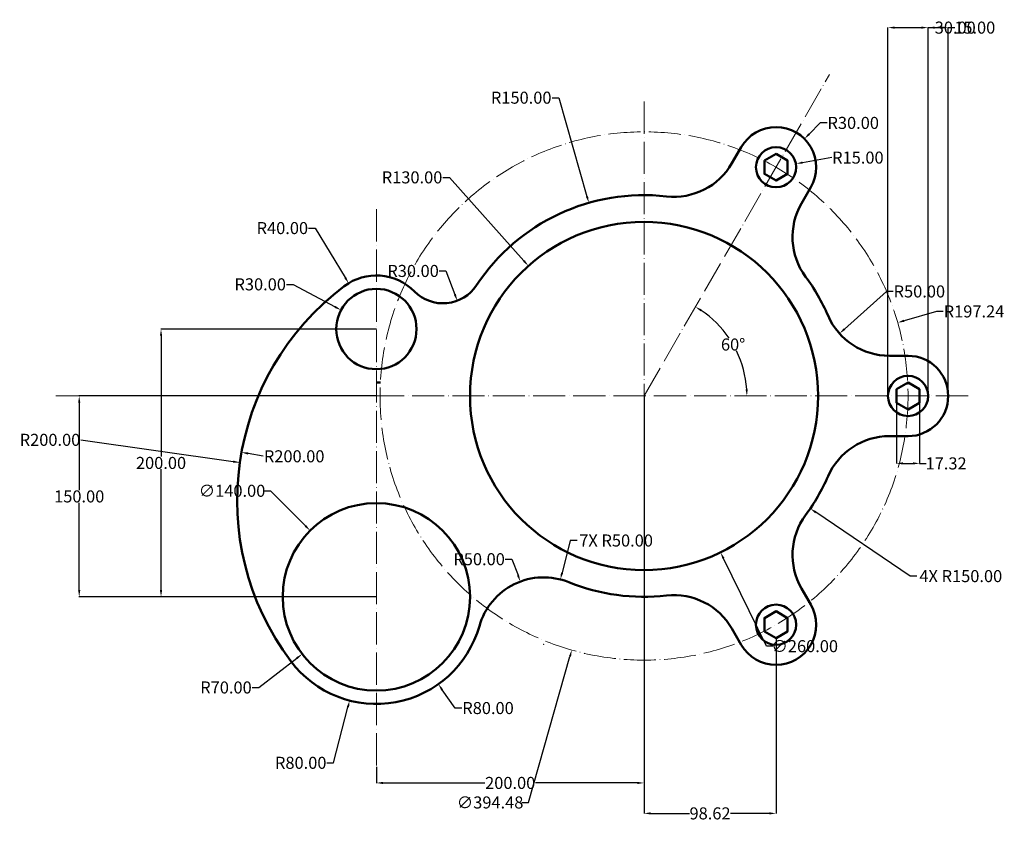
# Model space of a CAD drawing. Units: inches. Extents: x 301 to 1037, y 121 to 719.
import ezdxf

# ---------------------------------------------------------------- set-up
doc = ezdxf.new("R2010")
doc.units = ezdxf.units.IN
doc.header["$MEASUREMENT"] = 0
doc.linetypes.add('ACAD_ISO04W100', pattern=[30, 24, -3, 0, -3])
for name, color, linetype, lineweight in [('M-CNTR', 4, 'ACAD_ISO04W100', 18), ('M-DIMS', 2, 'Continuous', 25), ('M-OUTL', 7, 'Continuous', 50)]:
    doc.layers.add(name, color=color, linetype=linetype, lineweight=lineweight)
doc.styles.get("Standard").update_dxf_attribs({"font": 'arial.ttf'})
doc.dimstyles.get("Standard").update_dxf_attribs({"dimtxt": 9, "dimasz": 5, "dimexe": 0.18, "dimexo": 0.0625, "dimgap": 0.09, "dimtad": 0, "dimtih": 1, "dimtoh": 1, "dimzin": 0, "dimdsep": 46, "dimtxsty": 'Standard', "dimcen": 0.09, "dimadec": 0, "dimazin": 0, "dimtfac": 1, "dimtofl": 0, "dimtmove": 0, "dimatfit": 3, "dimfxl": 1, "dimtolj": 1, "dimtzin": 0, "dimarcsym": 0})

# ---------------------------------------------------------------- blocks, each defined once
blk = doc.blocks.new('*D1')
at = {"layer": 'Defpoints', "color": 0, "transparency": 16777216}
for p in [(567.87, 488.37), (406.98, 288.37), (567.87, 288.37)]:
    blk.add_point(p, dxfattribs=at)
at = {"layer": 'M-DIMS', "color": 0, "lineweight": -2, "transparency": 16777216}
for p, q in [((567.81, 488.37), (406.8, 488.37)), ((406.98, 483.37), (406.98, 393.06)), ((406.98, 293.37), (406.98, 383.69)), ((567.81, 288.37), (406.8, 288.37))]:
    blk.add_line(p, q, dxfattribs=at)
at = {"layer": 'M-DIMS', "color": 0, "transparency": 16777216}
for points in [[(406.15, 483.37), (407.81, 483.37), (406.98, 488.37)], [(406.15, 293.37), (407.81, 293.37), (406.98, 288.37)]]:
    blk.add_solid(points, dxfattribs=at)
at = {"layer": 'M-DIMS', "color": 0, "transparency": 16777216, "insert": (406.98, 388.37), "char_height": 9, "attachment_point": 5}
blk.add_mtext('\\A1;200.00', dxfattribs=at)
blk = doc.blocks.new('*D2')
at = {"layer": 'Defpoints', "color": 0, "transparency": 16777216}
for p in [(567.87, 438.37), (345.86, 288.37), (567.87, 288.37)]:
    blk.add_point(p, dxfattribs=at)
at = {"layer": 'M-DIMS', "color": 0, "lineweight": -2, "transparency": 16777216}
for p, q in [((567.81, 438.37), (345.68, 438.37)), ((345.86, 433.37), (345.86, 368.06)), ((345.86, 293.37), (345.86, 358.69)), ((567.81, 288.37), (345.68, 288.37))]:
    blk.add_line(p, q, dxfattribs=at)
at = {"layer": 'M-DIMS', "color": 0, "transparency": 16777216}
for points in [[(345.03, 433.37), (346.69, 433.37), (345.86, 438.37)], [(345.03, 293.37), (346.69, 293.37), (345.86, 288.37)]]:
    blk.add_solid(points, dxfattribs=at)
at = {"layer": 'M-DIMS', "color": 0, "transparency": 16777216, "insert": (345.86, 363.37), "char_height": 9, "attachment_point": 5}
blk.add_mtext('\\A1;150.00', dxfattribs=at)
blk = doc.blocks.new('*D3')
at = {"layer": 'Defpoints', "color": 0, "transparency": 16777216}
for p in [(567.87, 288.37), (512.43, 245.64)]:
    blk.add_point(p, dxfattribs=at)
at = {"layer": 'M-DIMS', "color": 0, "lineweight": -2, "transparency": 16777216}
for p, q in [((567.78, 288.37), (567.96, 288.37)), ((567.87, 288.28), (567.87, 288.46)), ((480.08, 220.7), (508.47, 242.58)), ((475.08, 220.7), (480.08, 220.7))]:
    blk.add_line(p, q, dxfattribs=at)
at = {"layer": 'M-DIMS', "color": 0, "transparency": 16777216}
blk.add_solid([(507.96, 243.24), (508.98, 241.92), (512.43, 245.64)], dxfattribs=at)
at = {"layer": 'M-DIMS', "color": 0, "transparency": 16777216, "insert": (455.51, 220.7), "char_height": 9, "attachment_point": 5}
blk.add_mtext('\\A1;R70.00', dxfattribs=at)
blk = doc.blocks.new('*D4')
at = {"layer": 'Defpoints', "color": 0, "transparency": 16777216}
for p in [(567.87, 288.37), (614.13, 223.11)]:
    blk.add_point(p, dxfattribs=at)
at = {"layer": 'M-DIMS', "color": 0, "lineweight": -2, "transparency": 16777216}
for p, q in [((567.78, 288.37), (567.96, 288.37)), ((567.87, 288.28), (567.87, 288.46)), ((626.73, 205.33), (617.02, 219.03)), ((631.73, 205.33), (626.73, 205.33))]:
    blk.add_line(p, q, dxfattribs=at)
at = {"layer": 'M-DIMS', "color": 0, "transparency": 16777216}
blk.add_solid([(617.7, 219.51), (616.34, 218.55), (614.13, 223.11)], dxfattribs=at)
at = {"layer": 'M-DIMS', "color": 0, "transparency": 16777216, "insert": (651.3, 205.33), "char_height": 9, "attachment_point": 5}
blk.add_mtext('\\A1;R80.00', dxfattribs=at)
blk = doc.blocks.new('*D5')
at = {"layer": 'Defpoints', "color": 0, "transparency": 16777216}
for p in [(767.87, 203.81), (567.87, 161.57), (767.87, 149.41)]:
    blk.add_point(p, dxfattribs=at)
at = {"layer": 'M-DIMS', "color": 0, "lineweight": -2, "transparency": 16777216}
for p, q in [((767.87, 203.75), (767.87, 149.23)), ((567.87, 161.51), (567.87, 149.23)), ((572.87, 149.41), (649.04, 149.41)), ((762.87, 149.41), (686.7, 149.41))]:
    blk.add_line(p, q, dxfattribs=at)
at = {"layer": 'M-DIMS', "color": 0, "transparency": 16777216}
for points in [[(572.87, 150.24), (572.87, 148.57), (567.87, 149.41)], [(762.87, 150.24), (762.87, 148.57), (767.87, 149.41)]]:
    blk.add_solid(points, dxfattribs=at)
at = {"layer": 'M-DIMS', "color": 0, "transparency": 16777216, "insert": (667.87, 149.41), "char_height": 9, "attachment_point": 5}
blk.add_mtext('\\A1;200.00', dxfattribs=at)
blk = doc.blocks.new('*D6')
at = {"layer": 'Defpoints', "color": 0, "transparency": 16777216}
for p in [(675.45, 299.77), (692.95, 252.94)]:
    blk.add_point(p, dxfattribs=at)
at = {"layer": 'M-DIMS', "color": 0, "lineweight": -2, "transparency": 16777216}
for p, q in [((664.2, 316.49), (669.2, 316.49)), ((669.2, 316.49), (673.7, 304.46)), ((692.86, 252.94), (693.04, 252.94)), ((692.95, 252.85), (692.95, 253.03))]:
    blk.add_line(p, q, dxfattribs=at)
at = {"layer": 'M-DIMS', "color": 0, "transparency": 16777216}
blk.add_solid([(674.48, 304.75), (672.92, 304.17), (675.45, 299.77)], dxfattribs=at)
at = {"layer": 'M-DIMS', "color": 0, "transparency": 16777216, "insert": (644.64, 316.49), "char_height": 9, "attachment_point": 5}
blk.add_mtext('\\A1;R50.00', dxfattribs=at)
blk = doc.blocks.new('*D7')
at = {"layer": 'Defpoints', "color": 0, "transparency": 16777216}
for p in [(541.43, 502.55), (567.87, 488.37)]:
    blk.add_point(p, dxfattribs=at)
at = {"layer": 'M-DIMS', "color": 0, "lineweight": -2, "transparency": 16777216}
for p, q in [((500.64, 521.73), (505.64, 521.73)), ((505.64, 521.73), (537.02, 504.91)), ((567.78, 488.37), (567.96, 488.37)), ((567.87, 488.28), (567.87, 488.46))]:
    blk.add_line(p, q, dxfattribs=at)
blk.add_arc((567.87, 488.37), 30, 151.46431, 224.53097, dxfattribs=at)
at = {"layer": 'M-DIMS', "color": 0, "transparency": 16777216}
blk.add_solid([(537.42, 505.64), (536.63, 504.17), (541.43, 502.55)], dxfattribs=at)
at = {"layer": 'M-DIMS', "color": 0, "transparency": 16777216, "insert": (481.07, 521.73), "char_height": 9, "attachment_point": 5}
blk.add_mtext('\\A1;R30.00', dxfattribs=at)
blk = doc.blocks.new('*D8')
at = {"layer": 'Defpoints', "color": 0, "transparency": 16777216}
for p in [(547.14, 522.58), (567.87, 488.37)]:
    blk.add_point(p, dxfattribs=at)
at = {"layer": 'M-DIMS', "color": 0, "lineweight": -2, "transparency": 16777216}
for p, q in [((517.2, 563.75), (522.2, 563.75)), ((522.2, 563.75), (544.55, 526.86)), ((567.78, 488.37), (567.96, 488.37)), ((567.87, 488.28), (567.87, 488.46))]:
    blk.add_line(p, q, dxfattribs=at)
at = {"layer": 'M-DIMS', "color": 0, "transparency": 16777216}
blk.add_solid([(545.26, 527.29), (543.84, 526.43), (547.14, 522.58)], dxfattribs=at)
at = {"layer": 'M-DIMS', "color": 0, "transparency": 16777216, "insert": (497.63, 563.75), "char_height": 9, "attachment_point": 5}
blk.add_mtext('\\A1;R40.00', dxfattribs=at)
blk = doc.blocks.new('*D9')
at = {"layer": 'Defpoints', "color": 0, "transparency": 16777216}
for p in [(617.67, 537.57), (628.28, 509.51)]:
    blk.add_point(p, dxfattribs=at)
at = {"layer": 'M-DIMS', "color": 0, "lineweight": -2, "transparency": 16777216}
for p, q in [((614.87, 531.74), (619.87, 531.74)), ((619.87, 531.74), (626.51, 514.18))]:
    blk.add_line(p, q, dxfattribs=at)
at = {"layer": 'M-DIMS', "color": 0, "transparency": 16777216}
blk.add_solid([(627.29, 514.48), (625.73, 513.89), (628.28, 509.51)], dxfattribs=at)
at = {"layer": 'M-DIMS', "color": 0, "transparency": 16777216, "insert": (595.3, 531.74), "char_height": 9, "attachment_point": 5}
blk.add_mtext('\\A1;R30.00', dxfattribs=at)
blk = doc.blocks.new('*D10')
at = {"layer": 'Defpoints', "color": 0, "transparency": 16777216}
for p in [(681.45, 535.49), (767.87, 438.37)]:
    blk.add_point(p, dxfattribs=at)
at = {"layer": 'M-DIMS', "color": 0, "lineweight": -2, "transparency": 16777216}
for p, q in [((617.6, 601.62), (622.6, 601.62)), ((622.6, 601.62), (678.13, 539.22)), ((767.78, 438.37), (767.96, 438.37)), ((767.87, 438.28), (767.87, 438.46))]:
    blk.add_line(p, q, dxfattribs=at)
at = {"layer": 'M-DIMS', "color": 0, "transparency": 16777216}
blk.add_solid([(678.75, 539.78), (677.5, 538.67), (681.45, 535.49)], dxfattribs=at)
at = {"layer": 'M-DIMS', "color": 0, "transparency": 16777216, "insert": (594.54, 601.62), "char_height": 9, "attachment_point": 5}
blk.add_mtext('\\A1;R130.00', dxfattribs=at)
blk = doc.blocks.new('*D11')
at = {"layer": 'Defpoints', "color": 0, "transparency": 16777216}
for p in [(467.12, 396.31), (663.87, 360.37)]:
    blk.add_point(p, dxfattribs=at)
at = {"layer": 'M-DIMS', "color": 0, "lineweight": -2, "transparency": 16777216}
blk.add_line((483.41, 393.33), (472.04, 395.41), dxfattribs=at)
at = {"layer": 'M-DIMS', "color": 0, "transparency": 16777216}
blk.add_solid([(472.19, 396.23), (471.89, 394.59), (467.12, 396.31)], dxfattribs=at)
at = {"layer": 'M-DIMS', "color": 0, "transparency": 16777216, "insert": (506.47, 393.33), "char_height": 9, "attachment_point": 5}
blk.add_mtext('\\A1;R200.00', dxfattribs=at)
blk = doc.blocks.new('*D12')
at = {"layer": 'Defpoints', "color": 0, "transparency": 16777216}
for p in [(726.62, 582.59), (767.87, 438.37)]:
    blk.add_point(p, dxfattribs=at)
at = {"layer": 'M-DIMS', "color": 0, "lineweight": -2, "transparency": 16777216}
for p, q in [((699.15, 661.13), (704.15, 661.13)), ((704.15, 661.13), (725.24, 587.4)), ((767.78, 438.37), (767.96, 438.37)), ((767.87, 438.28), (767.87, 438.46))]:
    blk.add_line(p, q, dxfattribs=at)
at = {"layer": 'M-DIMS', "color": 0, "transparency": 16777216}
blk.add_solid([(726.05, 587.63), (724.44, 587.17), (726.62, 582.59)], dxfattribs=at)
at = {"layer": 'M-DIMS', "color": 0, "transparency": 16777216, "insert": (676.09, 661.13), "char_height": 9, "attachment_point": 5}
blk.add_mtext('\\A1;R150.00', dxfattribs=at)
blk = doc.blocks.new('*U13')
for p, q in [((-0.06, 40.88), (-7.03, 28.81)), ((51.9, 10.88), (44.93, -1.19))]:
    blk.add_line(p, q)
blk.add_circle((25.92, 25.88), 15)
for centre, radius, start, end in [((25.92, 25.88), 30, 330, 150), ((-50.33, 53.81), 50, 263.57818, 330), ((88.23, -26.19), 50, 150, 216.42182)]:
    blk.add_arc(centre, radius, start, end)
blk = doc.blocks.new('*U14')
at = {"layer": 'M-OUTL', "color": 0, "linetype": 'ByBlock', "lineweight": -2, "transparency": 16777216}
blk.add_blockref('*U13', (840.57, 583.31), dxfattribs=at)
for p, rotation in [((929.74, 447.88), 300), ((857.04, 302.95), 240)]:
    blk.add_blockref('*U13', p, dxfattribs=dict(at, rotation=rotation))
blk = doc.blocks.new('*D15')
at = {"layer": 'Defpoints', "color": 0, "transparency": 16777216}
for p in [(956.45, 433.37), (973.77, 433.37), (973.77, 388.03)]:
    blk.add_point(p, dxfattribs=at)
at = {"layer": 'M-DIMS', "color": 0, "lineweight": -2, "transparency": 16777216}
for p, q in [((956.45, 433.31), (956.45, 387.85)), ((973.77, 433.31), (973.77, 387.85)), ((961.45, 388.03), (968.77, 388.03)), ((973.77, 388.03), (978.77, 388.03))]:
    blk.add_line(p, q, dxfattribs=at)
at = {"layer": 'M-DIMS', "color": 0, "transparency": 16777216}
for points in [[(961.45, 388.86), (961.45, 387.2), (956.45, 388.03)], [(968.77, 388.86), (968.77, 387.2), (973.77, 388.03)]]:
    blk.add_solid(points, dxfattribs=at)
at = {"layer": 'M-DIMS', "color": 0, "transparency": 16777216, "insert": (993.57, 388.03), "char_height": 9, "attachment_point": 5}
blk.add_mtext('\\A1;17.32', dxfattribs=at)
blk = doc.blocks.new('*D16')
at = {"layer": 'Defpoints', "color": 0, "transparency": 16777216}
for p in [(957.35, 493.14), (767.87, 438.37)]:
    blk.add_point(p, dxfattribs=at)
at = {"layer": 'M-DIMS', "color": 0, "lineweight": -2, "transparency": 16777216}
for p, q in [((986.35, 501.52), (962.16, 494.53)), ((991.35, 501.52), (986.35, 501.52)), ((767.78, 438.37), (767.96, 438.37)), ((767.87, 438.28), (767.87, 438.46))]:
    blk.add_line(p, q, dxfattribs=at)
at = {"layer": 'M-DIMS', "color": 0, "transparency": 16777216}
blk.add_solid([(961.92, 495.33), (962.39, 493.73), (957.35, 493.14)], dxfattribs=at)
at = {"layer": 'M-DIMS', "color": 0, "transparency": 16777216, "insert": (1014.41, 501.52), "char_height": 9, "attachment_point": 5}
blk.add_mtext('\\A1;R197.24', dxfattribs=at)
blk = doc.blocks.new('*D17')
at = {"layer": 'Defpoints', "color": 0, "transparency": 16777216}
for p in [(951.17, 518.37), (913.94, 485.01)]:
    blk.add_point(p, dxfattribs=at)
at = {"layer": 'M-DIMS', "color": 0, "lineweight": -2, "transparency": 16777216}
for p, q in [((949.01, 516.43), (917.66, 488.34)), ((954.01, 516.43), (949.01, 516.43))]:
    blk.add_line(p, q, dxfattribs=at)
at = {"layer": 'M-DIMS', "color": 0, "transparency": 16777216}
blk.add_solid([(917.1, 488.96), (918.21, 487.72), (913.94, 485.01)], dxfattribs=at)
at = {"layer": 'M-DIMS', "color": 0, "transparency": 16777216, "insert": (973.57, 516.43), "char_height": 9, "attachment_point": 5}
blk.add_mtext('\\A1;R50.00', dxfattribs=at)
blk = doc.blocks.new('*D18')
at = {"layer": 'Defpoints', "color": 0, "transparency": 16777216}
for p in [(887.7, 630.41), (866.49, 609.19)]:
    blk.add_point(p, dxfattribs=at)
at = {"layer": 'M-DIMS', "color": 0, "lineweight": -2, "transparency": 16777216}
for p, q in [((899.58, 642.3), (891.23, 633.94)), ((904.58, 642.3), (899.58, 642.3)), ((866.4, 609.19), (866.58, 609.19)), ((866.49, 609.1), (866.49, 609.28))]:
    blk.add_line(p, q, dxfattribs=at)
at = {"layer": 'M-DIMS', "color": 0, "transparency": 16777216}
blk.add_solid([(890.64, 634.53), (891.82, 633.35), (887.7, 630.41)], dxfattribs=at)
at = {"layer": 'M-DIMS', "color": 0, "transparency": 16777216, "insert": (924.15, 642.3), "char_height": 9, "attachment_point": 5}
blk.add_mtext('\\A1;R30.00', dxfattribs=at)
blk = doc.blocks.new('*D19')
at = {"layer": 'Defpoints', "color": 0, "transparency": 16777216}
for p in [(881.27, 611.74), (866.49, 609.19)]:
    blk.add_point(p, dxfattribs=at)
at = {"layer": 'M-DIMS', "color": 0, "lineweight": -2, "transparency": 16777216}
for p, q in [((908.06, 616.38), (886.2, 612.6)), ((866.4, 609.19), (866.58, 609.19)), ((866.49, 609.1), (866.49, 609.28))]:
    blk.add_line(p, q, dxfattribs=at)
at = {"layer": 'M-DIMS', "color": 0, "transparency": 16777216}
blk.add_solid([(886.05, 613.42), (886.34, 611.77), (881.27, 611.74)], dxfattribs=at)
at = {"layer": 'M-DIMS', "color": 0, "transparency": 16777216, "insert": (927.63, 616.38), "char_height": 9, "attachment_point": 5}
blk.add_mtext('\\A1;R15.00', dxfattribs=at)
blk = doc.blocks.new('*D20')
at = {"layer": 'Defpoints', "color": 0, "transparency": 16777216}
for p in [(906.54, 678.55), (840.09, 464.66), (328.38, 438.37), (767.87, 438.37), (1009.94, 438.37)]:
    blk.add_point(p, dxfattribs=at)
at = {"layer": 'M-DIMS', "color": 0, "lineweight": -2, "transparency": 16777216}
for start, end in [(34.12254, 56.27159), (3.72841, 26.04235)]:
    blk.add_arc((767.87, 438.37), 76.85, start, end, dxfattribs=at)
at = {"layer": 'M-DIMS', "color": 0, "transparency": 16777216}
for points in [[(810.1, 501.58), (810.98, 503), (806.29, 504.93)], [(845.39, 443.4), (843.72, 443.34), (844.72, 438.37)]]:
    blk.add_solid(points, dxfattribs=at)
at = {"layer": 'M-DIMS', "color": 0, "transparency": 16777216, "insert": (834.42, 476.8), "char_height": 9, "attachment_point": 5}
blk.add_mtext('\\A1;60°', dxfattribs=at)
blk = doc.blocks.new('*U21')
blk.add_lwpolyline([(8.66, 5), (0, 10), (-8.66, 5), (-8.66, -5), (0, -10), (8.66, -5)], close=True)
blk = doc.blocks.new('*U22')
at = {"layer": 'M-OUTL', "color": 0, "linetype": 'ByBlock', "lineweight": -2, "transparency": 16777216, "rotation": 60}
blk.add_blockref('*U21', (866.49, 609.19), dxfattribs=at)
at = {"layer": 'M-OUTL', "color": 0, "linetype": 'ByBlock', "lineweight": -2, "transparency": 16777216}
blk.add_blockref('*U21', (965.11, 438.37), dxfattribs=at)
blk = doc.blocks.new('*D23')
at = {"layer": 'Defpoints', "color": 0, "transparency": 16777216}
for p in [(980.11, 713.45), (950.11, 438.37), (980.11, 438.37)]:
    blk.add_point(p, dxfattribs=at)
at = {"layer": 'M-DIMS', "color": 0, "lineweight": -2, "transparency": 16777216}
for p, q in [((950.11, 438.44), (950.11, 713.63)), ((980.11, 438.44), (980.11, 713.63)), ((955.11, 713.45), (975.11, 713.45)), ((980.11, 713.45), (985.11, 713.45))]:
    blk.add_line(p, q, dxfattribs=at)
at = {"layer": 'M-DIMS', "color": 0, "transparency": 16777216}
for points in [[(955.11, 714.29), (955.11, 712.62), (950.11, 713.45)], [(975.11, 714.29), (975.11, 712.62), (980.11, 713.45)]]:
    blk.add_solid(points, dxfattribs=at)
at = {"layer": 'M-DIMS', "color": 0, "transparency": 16777216, "insert": (1000.37, 713.45), "char_height": 9, "attachment_point": 5}
blk.add_mtext('\\A1;30.00', dxfattribs=at)
blk = doc.blocks.new('*D24')
at = {"layer": 'Defpoints', "color": 0, "transparency": 16777216}
for p in [(995.11, 713.45), (980.11, 438.37), (995.11, 438.37)]:
    blk.add_point(p, dxfattribs=at)
at = {"layer": 'M-DIMS', "color": 0, "lineweight": -2, "transparency": 16777216}
for p, q in [((980.11, 438.44), (980.11, 713.63)), ((995.11, 438.44), (995.11, 713.63)), ((985.11, 713.45), (990.11, 713.45)), ((995.11, 713.45), (1000.11, 713.45))]:
    blk.add_line(p, q, dxfattribs=at)
at = {"layer": 'M-DIMS', "color": 0, "transparency": 16777216}
for points in [[(985.11, 714.29), (985.11, 712.62), (980.11, 713.45)], [(990.11, 714.29), (990.11, 712.62), (995.11, 713.45)]]:
    blk.add_solid(points, dxfattribs=at)
at = {"layer": 'M-DIMS', "color": 0, "transparency": 16777216, "insert": (1014.95, 713.45), "char_height": 9, "attachment_point": 5}
blk.add_mtext('\\A1;15.00', dxfattribs=at)
blk = doc.blocks.new('*D25')
at = {"layer": 'Defpoints', "color": 0, "transparency": 16777216}
for p in [(767.87, 438.37), (866.49, 257.56), (866.49, 126.67)]:
    blk.add_point(p, dxfattribs=at)
at = {"layer": 'M-DIMS', "color": 0, "lineweight": -2, "transparency": 16777216}
for p, q in [((767.87, 438.31), (767.87, 126.49)), ((866.49, 257.5), (866.49, 126.49)), ((772.87, 126.67), (801.95, 126.67)), ((861.49, 126.67), (832.41, 126.67))]:
    blk.add_line(p, q, dxfattribs=at)
at = {"layer": 'M-DIMS', "color": 0, "transparency": 16777216}
for points in [[(772.87, 127.5), (772.87, 125.83), (767.87, 126.67)], [(861.49, 127.5), (861.49, 125.83), (866.49, 126.67)]]:
    blk.add_solid(points, dxfattribs=at)
at = {"layer": 'M-DIMS', "color": 0, "transparency": 16777216, "insert": (817.18, 126.67), "char_height": 9, "attachment_point": 5}
blk.add_mtext('\\A1;98.62', dxfattribs=at)
blk = doc.blocks.new('*D26')
at = {"layer": 'Defpoints', "color": 0, "transparency": 16777216}
for p in [(710.74, 555.15), (825, 321.6)]:
    blk.add_point(p, dxfattribs=at)
at = {"layer": 'M-DIMS', "color": 0, "lineweight": -2, "transparency": 16777216}
for p, q in [((767.78, 438.37), (767.96, 438.37)), ((767.87, 438.28), (767.87, 438.46)), ((859.28, 251.54), (827.2, 317.11)), ((864.28, 251.54), (859.28, 251.54))]:
    blk.add_line(p, q, dxfattribs=at)
at = {"layer": 'M-DIMS', "color": 0, "transparency": 16777216}
blk.add_solid([(827.95, 317.47), (826.45, 316.74), (825, 321.6)], dxfattribs=at)
at = {"layer": 'M-DIMS', "color": 0, "transparency": 16777216, "insert": (887.93, 251.54), "char_height": 9, "attachment_point": 5}
blk.add_mtext('\\A1;∅260.00', dxfattribs=at)
blk = doc.blocks.new('*D27')
at = {"layer": 'Defpoints', "color": 0, "transparency": 16777216}
for p in [(518.37, 337.87), (617.37, 238.88)]:
    blk.add_point(p, dxfattribs=at)
at = {"layer": 'M-DIMS', "color": 0, "lineweight": -2, "transparency": 16777216}
for p, q in [((483.67, 367.57), (488.67, 367.57)), ((488.67, 367.57), (514.84, 341.4)), ((567.78, 288.37), (567.96, 288.37)), ((567.87, 288.28), (567.87, 288.46))]:
    blk.add_line(p, q, dxfattribs=at)
at = {"layer": 'M-DIMS', "color": 0, "transparency": 16777216}
blk.add_solid([(515.42, 341.99), (514.25, 340.82), (518.37, 337.87)], dxfattribs=at)
at = {"layer": 'M-DIMS', "color": 0, "transparency": 16777216, "insert": (460.02, 367.57), "char_height": 9, "attachment_point": 5}
blk.add_mtext('\\A1;∅140.00', dxfattribs=at)
blk = doc.blocks.new('*D28')
at = {"layer": 'Defpoints', "color": 0, "transparency": 16777216}
for p in [(465.88, 388.66), (663.87, 360.37)]:
    blk.add_point(p, dxfattribs=at)
at = {"layer": 'M-DIMS', "color": 0, "lineweight": -2, "transparency": 16777216}
for p, q in [((347.09, 405.63), (460.93, 389.36)), ((663.78, 360.37), (663.96, 360.37)), ((663.87, 360.28), (663.87, 360.46))]:
    blk.add_line(p, q, dxfattribs=at)
at = {"layer": 'M-DIMS', "color": 0, "transparency": 16777216}
blk.add_solid([(461.05, 390.19), (460.81, 388.54), (465.88, 388.66)], dxfattribs=at)
at = {"layer": 'M-DIMS', "color": 0, "transparency": 16777216, "insert": (324.02, 405.63), "char_height": 9, "attachment_point": 5}
blk.add_mtext('\\A1;R200.00', dxfattribs=at)
blk = doc.blocks.new('*D29')
at = {"layer": 'Defpoints', "color": 0, "transparency": 16777216}
for p in [(821.84, 628.09), (713.9, 248.66)]:
    blk.add_point(p, dxfattribs=at)
at = {"layer": 'M-DIMS', "color": 0, "lineweight": -2, "transparency": 16777216}
for p, q in [((767.78, 438.37), (767.96, 438.37)), ((767.87, 438.28), (767.87, 438.46)), ((681.52, 134.83), (712.53, 243.85)), ((676.52, 134.83), (681.52, 134.83))]:
    blk.add_line(p, q, dxfattribs=at)
at = {"layer": 'M-DIMS', "color": 0, "transparency": 16777216}
blk.add_solid([(711.73, 244.08), (713.33, 243.62), (713.9, 248.66)], dxfattribs=at)
at = {"layer": 'M-DIMS', "color": 0, "transparency": 16777216, "insert": (652.84, 134.83), "char_height": 9, "attachment_point": 5}
blk.add_mtext('\\A1;∅394.48', dxfattribs=at)
blk = doc.blocks.new('*D30')
at = {"layer": 'Defpoints', "color": 0, "transparency": 16777216}
for p in [(767.87, 438.37), (892.1, 354.3)]:
    blk.add_point(p, dxfattribs=at)
at = {"layer": 'M-DIMS', "color": 0, "lineweight": -2, "transparency": 16777216}
for p, q in [((767.78, 438.37), (767.96, 438.37)), ((767.87, 438.28), (767.87, 438.46)), ((966.63, 303.86), (896.24, 351.5)), ((971.63, 303.86), (966.63, 303.86))]:
    blk.add_line(p, q, dxfattribs=at)
at = {"layer": 'M-DIMS', "color": 0, "transparency": 16777216}
blk.add_solid([(896.7, 352.19), (895.77, 350.81), (892.1, 354.3)], dxfattribs=at)
at = {"layer": 'M-DIMS', "color": 0, "transparency": 16777216, "insert": (1004.54, 303.86), "char_height": 9, "attachment_point": 5}
blk.add_mtext('\\A1;4X R150.00', dxfattribs=at)
blk = doc.blocks.new('*D31')
at = {"layer": 'Defpoints', "color": 0, "transparency": 16777216}
for p in [(567.87, 288.37), (547.9, 210.91)]:
    blk.add_point(p, dxfattribs=at)
at = {"layer": 'M-DIMS', "color": 0, "lineweight": -2, "transparency": 16777216}
for p, q in [((567.78, 288.37), (567.96, 288.37)), ((567.87, 288.28), (567.87, 288.46)), ((535.92, 164.43), (546.65, 206.06)), ((530.92, 164.43), (535.92, 164.43))]:
    blk.add_line(p, q, dxfattribs=at)
at = {"layer": 'M-DIMS', "color": 0, "transparency": 16777216}
blk.add_solid([(545.84, 206.27), (547.46, 205.86), (547.9, 210.91)], dxfattribs=at)
at = {"layer": 'M-DIMS', "color": 0, "transparency": 16777216, "insert": (511.35, 164.43), "char_height": 9, "attachment_point": 5}
blk.add_mtext('\\A1;R80.00', dxfattribs=at)
blk = doc.blocks.new('*D32')
at = {"layer": 'Defpoints', "color": 0, "transparency": 16777216}
for p in [(705.35, 301.37), (692.95, 252.94)]:
    blk.add_point(p, dxfattribs=at)
at = {"layer": 'M-DIMS', "color": 0, "lineweight": -2, "transparency": 16777216}
for p, q in [((712.79, 330.44), (706.59, 306.22)), ((717.79, 330.44), (712.79, 330.44)), ((692.86, 252.94), (693.04, 252.94)), ((692.95, 252.85), (692.95, 253.03))]:
    blk.add_line(p, q, dxfattribs=at)
at = {"layer": 'M-DIMS', "color": 0, "transparency": 16777216}
blk.add_solid([(705.78, 306.42), (707.4, 306.01), (705.35, 301.37)], dxfattribs=at)
at = {"layer": 'M-DIMS', "color": 0, "transparency": 16777216, "insert": (746.99, 330.44), "char_height": 9, "attachment_point": 5}
blk.add_mtext('\\A1;7X R50.00', dxfattribs=at)

msp = doc.modelspace()

# ---------------------------------------------------------------- linework, layer by layer
at = {"layer": 'M-CNTR'}
for p, q in [((767.869, 438.373), (906.538, 678.554)), ((767.869, 658.245), (767.869, 203.811)), ((567.869, 577.82), (567.869, 161.568)), ((1009.939, 438.373), (328.382, 438.373))]:
    msp.add_line(p, q, dxfattribs=at)
msp.add_circle((767.869, 438.373), 197.24, dxfattribs=at)
at = {"layer": 'M-OUTL'}
msp.add_lwpolyline([(875.149, 272.558), (866.489, 277.558), (857.829, 272.558), (857.829, 262.558), (866.489, 257.558), (875.149, 262.558)], close=True, dxfattribs=at)
for centre, radius in [((767.869, 438.373), 130), ((567.869, 488.373), 30), ((567.869, 288.373), 70)]:
    msp.add_circle(centre, radius, dxfattribs=at)
for centre, radius, start, end in [((767.869, 438.373), 150, 83.578178, 146.558831), ((567.869, 488.373), 40, 44.650339, 126.869898), ((767.869, 438.373), 150, 23.578178, 36.421822), ((663.869, 360.373), 200, 126.869898, 216.869898), ((617.668, 537.567), 30, 224.650339, 326.558831), ((567.869, 488.373), 40, 270, 274.329217), ((767.869, 438.373), 150, 323.578178, 336.421822), ((692.946, 252.937), 50, 67.999511, 164.181815), ((767.869, 438.373), 150, 247.999511, 276.421822), ((567.869, 288.373), 80, 216.869898, 344.181815)]:
    msp.add_arc(centre, radius, start, end, dxfattribs=at)

# ---------------------------------------------------------------- block references
for name in ['*U14', '*U22']:
    msp.add_blockref(name, (0, 0), dxfattribs=at)

# ---------------------------------------------------------------- dimensions: what is measured, and where the dimension line sits
at = {"layer": 'M-DIMS'}
for base, p1, p2, override, picture, middle in [((980.109, 713.454), (950.109, 438.373), (980.109, 438.373), {"dimdec": 2, "dimlfac": 1, "dimrnd": 0, "dimzin": 0, "dimdsep": 46, "dimlunit": 2}, '*D23', (1000.366, 713.454)), ((995.109, 713.454), (980.109, 438.373), (995.109, 438.373), {"dimdec": 2, "dimlfac": 1, "dimrnd": 0, "dimzin": 0, "dimdsep": 46, "dimlunit": 2}, '*D24', (1014.946, 713.454)), ((866.489, 126.668), (767.869, 438.373), (866.489, 257.558), {"dimdec": 2, "dimlfac": 1, "dimrnd": 0, "dimzin": 0, "dimdsep": 46, "dimlunit": 2}, '*D25', (817.179, 126.668)), ((767.869, 149.407), (567.869, 161.568), (767.869, 203.811), {"dimclrd": 0, "dimclre": 0, "dimclrt": 0}, '*D5', (667.869, 149.407))]:
    dim = msp.add_linear_dim(base=base, p1=p1, p2=p2, dimstyle='Standard', override=override, dxfattribs=at)
    dim.commit()
    dim.dimension.update_dxf_attribs({"geometry": picture, "text_midpoint": middle})
dim = msp.add_angular_dim_2l(base=(840.085, 464.657), line1=((1009.939, 438.373), (328.382, 438.373)), line2=((767.869, 438.373), (906.538, 678.554)), dimstyle='Standard', override={"dimclrd": 0, "dimclre": 0, "dimclrt": 0}, dxfattribs=at)
dim.commit()
dim.dimension.update_dxf_attribs({"geometry": '*D20', "text_midpoint": (834.424, 476.798)})
for center, mpoint, override, picture, middle in [((767.869, 438.373), (726.619, 582.589), {"dimclrd": 0, "dimclre": 0, "dimclrt": 0}, '*D12', (676.09, 661.134)), ((866.489, 609.188), (887.697, 630.407), {"dimclrd": 0, "dimclre": 0, "dimclrt": 0}, '*D18', (924.15, 642.3)), ((866.489, 609.188), (881.27, 611.744), {"dimclrd": 0, "dimclre": 0, "dimclrt": 0}, '*D19', (908.059, 616.376)), ((767.869, 438.373), (681.45, 535.489), {"dimclrd": 0, "dimclre": 0, "dimclrt": 0}, '*D10', (594.541, 601.619)), ((567.869, 488.373), (547.142, 522.584), {"dimclrd": 0, "dimclre": 0, "dimclrt": 0}, '*D8', (497.635, 563.749)), ((617.668, 537.567), (628.277, 509.506), {"dimclrd": 0, "dimclre": 0, "dimclrt": 0}, '*D9', (595.304, 531.742)), ((567.869, 488.373), (541.428, 502.546), {"dimclrd": 0, "dimclre": 0, "dimclrt": 0}, '*D7', (481.075, 521.728)), ((951.172, 518.373), (913.935, 485.005), {"dimclrd": 0, "dimclre": 0, "dimclrt": 0}, '*D17', (973.572, 516.432)), ((767.869, 438.373), (957.353, 493.142), {"dimclrd": 0, "dimclre": 0, "dimclrt": 0}, '*D16', (1014.407, 501.523)), ((663.869, 360.373), (465.879, 388.657), {"dimdec": 2, "dimlfac": 1, "dimrnd": 0, "dimzin": 0, "dimdsep": 46, "dimlunit": 2}, '*D28', (347.085, 405.627)), ((663.869, 360.373), (467.124, 396.308), {"dimclrd": 0, "dimclre": 0, "dimclrt": 0}, '*D11', (483.408, 393.334)), ((692.946, 252.937), (675.447, 299.774), {"dimclrd": 0, "dimclre": 0, "dimclrt": 0}, '*D6', (644.636, 316.487)), ((567.869, 288.373), (512.429, 245.637), {"dimclrd": 0, "dimclre": 0, "dimclrt": 0}, '*D3', (455.511, 220.701)), ((567.869, 288.373), (547.899, 210.906), {"dimdec": 2, "dimlfac": 1, "dimrnd": 0, "dimzin": 0, "dimdsep": 46, "dimlunit": 2}, '*D31', (511.35, 164.425)), ((567.869, 288.373), (614.133, 223.107), {"dimclrd": 0, "dimclre": 0, "dimclrt": 0}, '*D4', (651.3, 205.33))]:
    dim = msp.add_radius_dim(center=center, mpoint=mpoint, dimstyle='Standard', override=override, dxfattribs=at)
    dim.commit()
    dim.dimension.update_dxf_attribs({"geometry": picture, "text_midpoint": middle, "dimtype": 164})
for p1, p2, picture, middle in [((821.839, 628.086), (713.9, 248.66), '*D29', (652.842, 134.832)), ((710.738, 555.146), (825, 321.599), '*D26', (887.931, 251.535)), ((617.368, 238.876), (518.371, 337.869), '*D27', (460.02, 367.567))]:
    dim = msp.add_diameter_dim_2p(p1=p1, p2=p2, dimstyle='Standard', override={"dimdec": 2, "dimlfac": 1, "dimrnd": 0, "dimzin": 0, "dimdsep": 46, "dimlunit": 2}, dxfattribs=at)
    dim.commit()
    dim.dimension.update_dxf_attribs({"geometry": picture, "text_midpoint": middle, "dimtype": 163})
for base, p1, p2, angle, picture, middle in [((406.981, 288.373), (567.869, 488.373), (567.869, 288.373), 90, '*D1', (406.981, 388.373)), ((345.862, 288.373), (567.869, 438.373), (567.869, 288.373), 90, '*D2', (345.862, 363.373)), ((973.769, 388.031), (956.449, 433.373), (973.769, 433.373), 0.000019, '*D15', (993.575, 388.031))]:
    dim = msp.add_linear_dim(base=base, p1=p1, p2=p2, angle=angle, dimstyle='Standard', override={"dimclrd": 0, "dimclre": 0, "dimclrt": 0}, dxfattribs=at)
    dim.commit()
    dim.dimension.update_dxf_attribs({"geometry": picture, "text_midpoint": middle})
for center, mpoint, text, picture, middle in [((767.869, 438.373), (892.096, 354.303), '4X <>', '*D30', (1004.545, 303.861)), ((692.946, 252.937), (705.352, 301.373), '7X <>', '*D32', (746.994, 330.435))]:
    dim = msp.add_radius_dim(center=center, mpoint=mpoint, text=text, dimstyle='Standard', override={"dimdec": 2, "dimlfac": 1, "dimrnd": 0, "dimzin": 0, "dimdsep": 46, "dimlunit": 2}, dxfattribs=at)
    dim.commit()
    dim.dimension.update_dxf_attribs({"geometry": picture, "text_midpoint": middle, "dimtype": 164})

doc.saveas('drawing.dxf')
